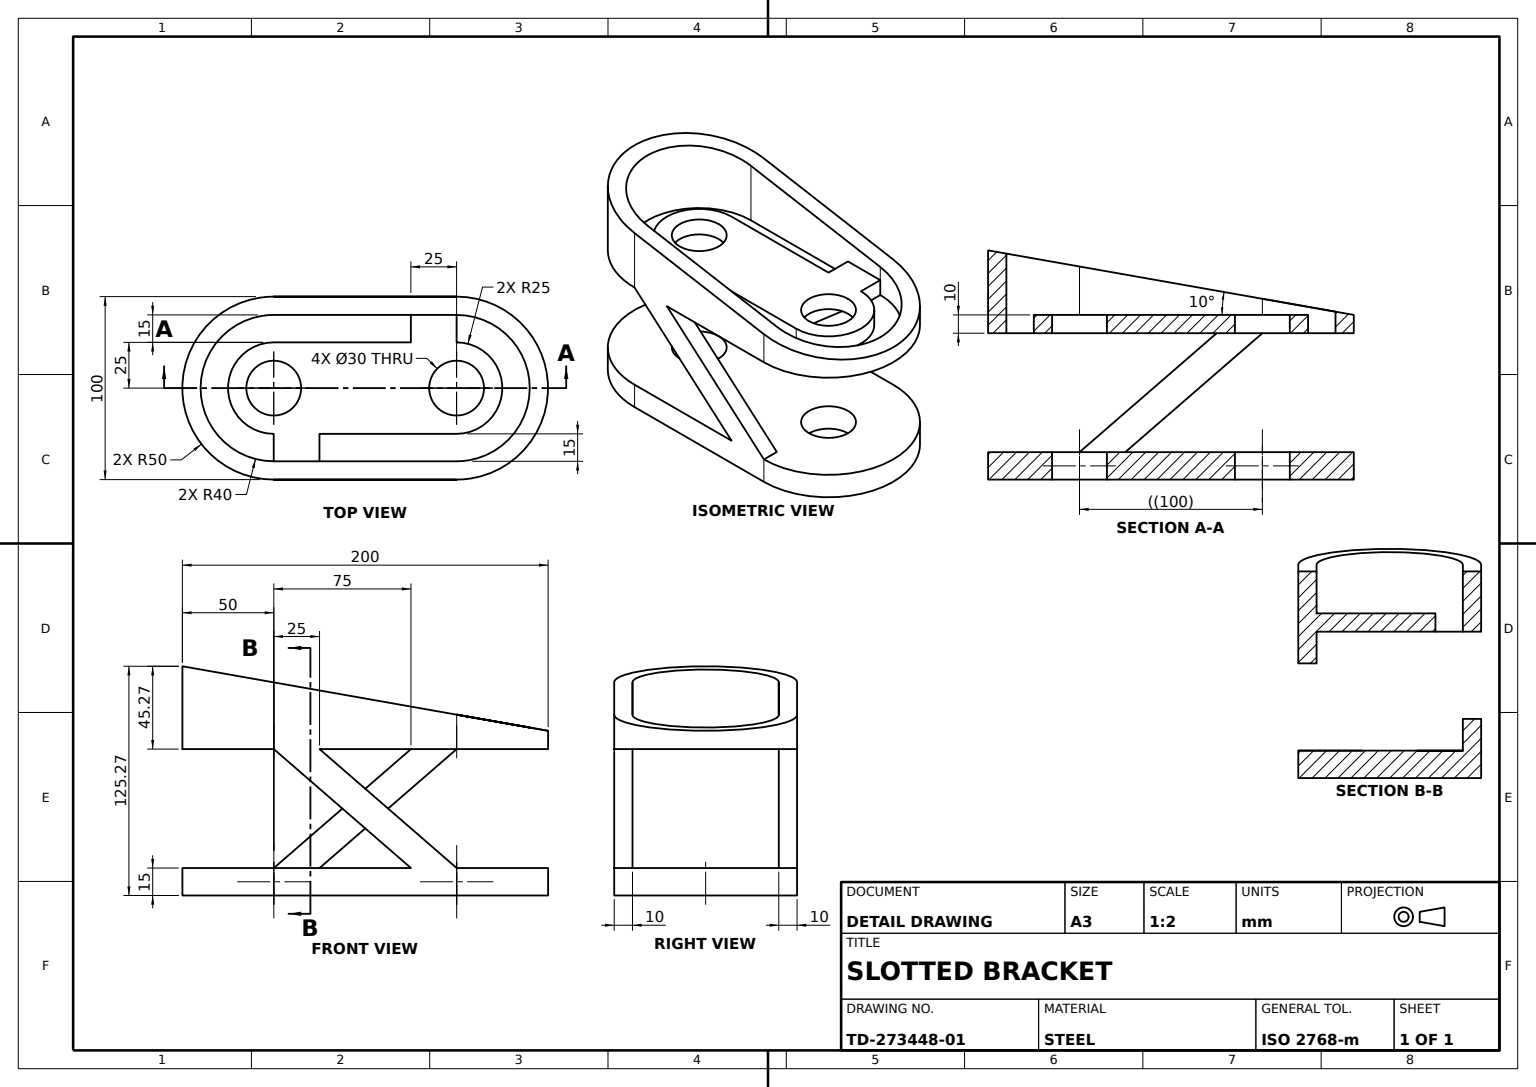
from build123d import *

# Parameters (mm, degrees)
BASE_PLATE_DEPTH            = 15
BASE_BORE_SKETCH_R          = 15
BASE_BORE_DEPTH             = 15
LOOP_START                  = -10
LOOP_RING_DEPTH             = 50
BRACE_ANGLE_CUT_DEPTH       = 223.261107709
X_BRACE_WEB_DEPTH           = 10
BRACE_TRIM_CUT_SKETCH_R     = 15
BRACE_TRIM_CUT_DEPTH        = 10
INNER_PLATE_DEPTH           = 10
INNER_PLATE_EXTENSION_DEPTH = 10


with BuildPart() as part:
    # Base Plate Sketch → Base Plate (new body)
    with BuildSketch(Plane(origin=(0, 0, 0), x_dir=(1, 0, 0), z_dir=(0, 1, 0))):
        with BuildLine():
            Line((0, 50), (100, 50))
            ThreePointArc((100, 50), (150, 0), (100, -50))
            Line((100, -50), (0, -50))
            ThreePointArc((0, -50), (-50, 0), (0, 50))
        make_face()
    extrude(amount=BASE_PLATE_DEPTH)

    # Base Bore Sketch → Base Bore (cut)
    with BuildSketch(Plane(origin=(0, 15, 0), x_dir=(1, 0, 0), z_dir=(0, 1, 0))):
        with Locations(Location((100, 0, 0), (0, 0, 270))):
            Circle(BASE_BORE_SKETCH_R)
        with Locations(Location((0, 0, 0), (0, 0, 270))):
            Circle(BASE_BORE_SKETCH_R)
    extrude(amount=-BASE_BORE_DEPTH, mode=Mode.SUBTRACT)



with BuildPart() as body_2:
    # Loop Ring Sketch → Loop Ring (new body)
    with BuildSketch(Plane(origin=(0, 90, 0), x_dir=(1, 0, 0), z_dir=(0, 1, 0)).offset(LOOP_START)):
        with BuildLine():
            Line((0, -50), (100, -50))
            ThreePointArc((100, -50), (150, 0), (100, 50))
            Line((100, 50), (0, 50))
            ThreePointArc((0, 50), (-50, 0), (0, -50))
        make_face()
        with BuildLine():
            Line((0, 40), (100, 40))
            ThreePointArc((100, 40), (140, 0), (100, -40))
            Line((100, -40), (0, -40))
            ThreePointArc((0, -40), (-40, 0), (0, 40))
        make_face(mode=Mode.SUBTRACT)
    extrude(amount=LOOP_RING_DEPTH)

    # Brace Angle Cut Sketch → Brace Angle Cut (cut, through all)
    with BuildSketch(Plane.XY.offset(50)):
        Polygon((150, 90), (150, 130), (-50, 130), (-50, 125.265396142), align=None)
    extrude(amount=-BRACE_ANGLE_CUT_DEPTH, mode=Mode.SUBTRACT)

    # X-Brace Sketch → X-Brace Web (add)
    with BuildSketch(Plane(origin=(0, 90, 0), x_dir=(1, 0, 0), z_dir=(0, 1, 0))):
        with BuildLine():
            Line((0, 25), (75, 25))
            Line((75, 25), (75, 40))
            Line((75, 40), (100, 40))
            Line((100, 40), (100, 25))
            ThreePointArc((100, 25), (125, 0), (100, -25))
            Line((100, -25), (25, -25))
            Line((25, -25), (25, -40))
            Line((25, -40), (0, -40))
            Line((0, -40), (0, -25))
            ThreePointArc((0, -25), (-25, 0), (0, 25))
        make_face()
    extrude(amount=-X_BRACE_WEB_DEPTH)

    # Brace Trim Cut Sketch → Brace Trim Cut (cut)
    with BuildSketch(Plane(origin=(0, 90, 0), x_dir=(1, 0, 0), z_dir=(0, 1, 0))):
        with Locations(Location((100, 0, 0), (0, 0, 270))):
            Circle(BRACE_TRIM_CUT_SKETCH_R)
        with Locations(Location((0, 0, 0), (0, 0, 270))):
            Circle(BRACE_TRIM_CUT_SKETCH_R)
    extrude(amount=-BRACE_TRIM_CUT_DEPTH, mode=Mode.SUBTRACT)


with BuildPart() as part_1:
    add(part.part)

    add(body_2.part)  # Inner Plate merges body 2
    # Inner Plate Sketch → Inner Plate (add)
    with BuildSketch(Plane.XY.offset(50)):
        Polygon((0, 80), (75, 15), (100, 15), (25, 80), align=None)
    extrude(amount=-INNER_PLATE_DEPTH)

    # Inner Plate Extension Sketch → Inner Plate Extension (add)
    with BuildSketch(Plane(origin=(0, 0, -50), x_dir=(-1, 0, 0), z_dir=(0, 0, -1))):
        Polygon((-100, 80), (-25, 15), (0, 15), (-75, 80), align=None)
    extrude(amount=-INNER_PLATE_EXTENSION_DEPTH)


solid = part_1.part
